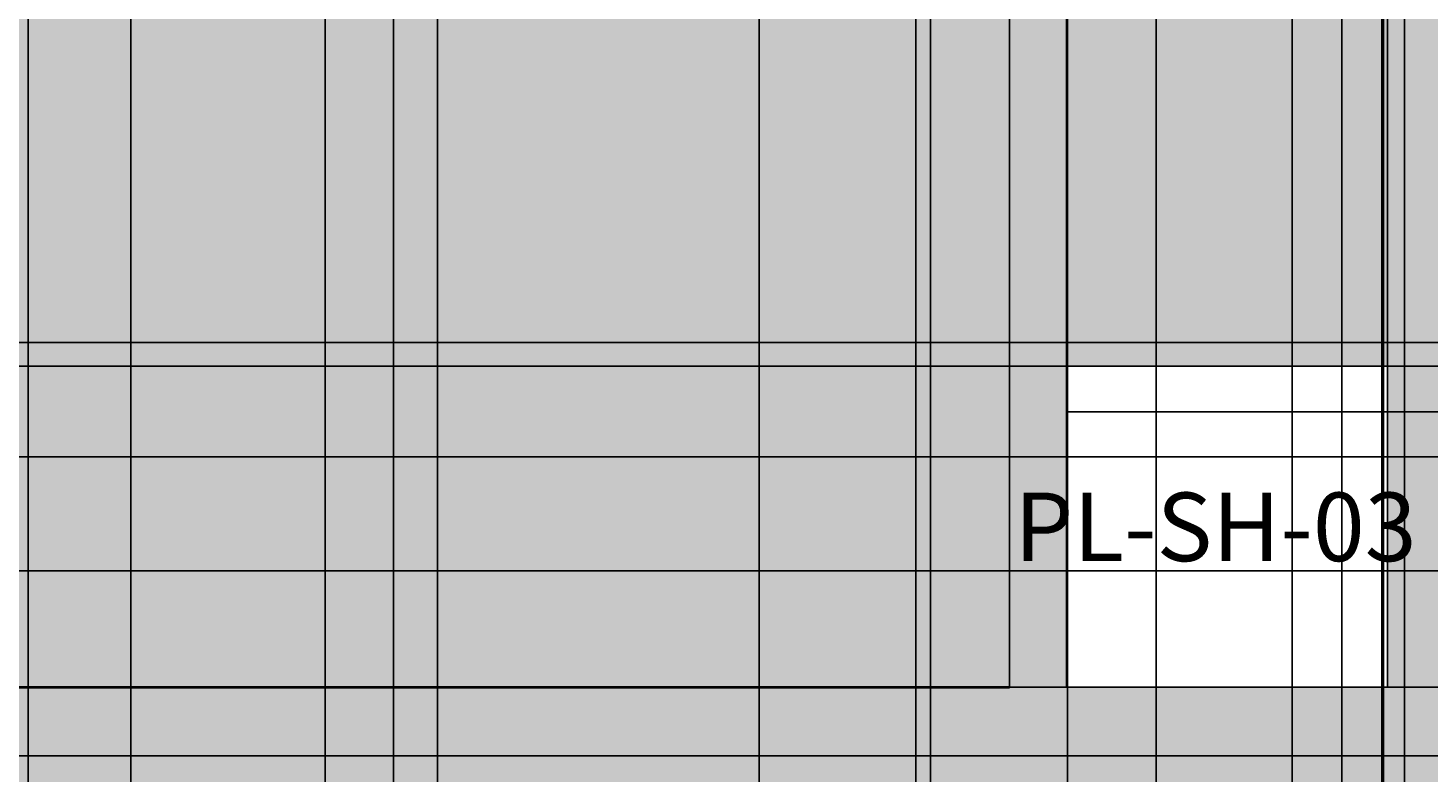
# Model space of a CAD drawing. Units: inches. Extents: x 818 to 1898, y 976 to 2364.
# Tile 91 of 96: x 1591 to 1713, y 2046 to 2111. Entities that reach past the tile are written whole.
import ezdxf

# ---------------------------------------------------------------- set-up
doc = ezdxf.new("R2010")
doc.units = ezdxf.units.IN
doc.header["$LTSCALE"] = 5
doc.header["$MEASUREMENT"] = 0
for name, color, linetype, lineweight in [('A-ANNO-DIMS', 2, 'Continuous', 18), ('A-ANNO-TEXT', 7, 'Continuous', 18), ('A-FLOR-SHFT', 7, 'Continuous', 25), ('A-WALL', 7, 'Continuous', 40)]:
    doc.layers.add(name, color=color, linetype=linetype, lineweight=lineweight)
doc.layers.add('A-WALL-PATT', color=251, linetype='Continuous', lineweight=13, true_color=0x636466)
doc.layers.add('L-PLNT-PATT', color=114, linetype='Continuous', lineweight=9, true_color=0x139b48)
doc.styles.get("Standard").update_dxf_attribs({"font": 'arial.ttf'})
doc.dimstyles.get("Standard").update_dxf_attribs({"dimtxt": 0.18, "dimasz": 0.18, "dimexe": 0.18, "dimexo": 0.0625, "dimgap": 0.09, "dimtad": 0, "dimtih": 1, "dimtoh": 1, "dimdec": 4, "dimzin": 0, "dimdsep": 46, "dimtxsty": 'Standard', "dimcen": 0.09, "dimadec": 0, "dimazin": 0, "dimtfac": 1, "dimtdec": 4, "dimtofl": 0, "dimtmove": 0, "dimatfit": 3, "dimfxl": 1, "dimtolj": 1, "dimtzin": 0, "dimarcsym": 0})

# ---------------------------------------------------------------- blocks, each defined once
blk = doc.blocks.new('*D85')
at = {"layer": 'A-ANNO-DIMS', "color": 0, "lineweight": -2, "ltscale": 5, "transparency": 16777216}
for p, q in [((1258.79, 2053.08), (1897.92, 2053.08)), ((1897.74, 2052.9), (1897.74, 1876.76)), ((1897.74, 1700.26), (1897.74, 1876.4)), ((1258.79, 1700.08), (1897.92, 1700.08))]:
    blk.add_line(p, q, dxfattribs=at)
at = {"layer": 'A-ANNO-DIMS', "color": 0, "ltscale": 5, "transparency": 16777216}
for points in [[(1897.71, 2052.9), (1897.77, 2052.9), (1897.74, 2053.08)], [(1897.71, 1700.26), (1897.77, 1700.26), (1897.74, 1700.08)]]:
    blk.add_solid(points, dxfattribs=at)
at = {"layer": 'Defpoints', "color": 0, "ltscale": 5, "transparency": 16777216}
for p in [(1258.73, 2053.08), (1897.74, 2053.08), (1258.73, 1700.08)]:
    blk.add_point(p, dxfattribs=at)
at = {"layer": 'A-ANNO-DIMS', "color": 0, "ltscale": 5, "transparency": 16777216, "insert": (1897.74, 1876.58), "char_height": 0.18, "attachment_point": 5}
blk.add_mtext('\\A1;353', dxfattribs=at)
blk = doc.blocks.new('*D86')
at = {"layer": 'A-ANNO-DIMS', "color": 0, "lineweight": -2, "ltscale": 5, "transparency": 16777216}
for p, q in [((1258.73, 2053.14), (1258.73, 2363.87)), ((1258.91, 2363.69), (1486.43, 2363.69)), ((1714.55, 2363.69), (1487.02, 2363.69)), ((1714.73, 2053.14), (1714.73, 2363.87))]:
    blk.add_line(p, q, dxfattribs=at)
at = {"layer": 'A-ANNO-DIMS', "color": 0, "ltscale": 5, "transparency": 16777216}
for points in [[(1258.91, 2363.72), (1258.91, 2363.66), (1258.73, 2363.69)], [(1714.55, 2363.72), (1714.55, 2363.66), (1714.73, 2363.69)]]:
    blk.add_solid(points, dxfattribs=at)
at = {"layer": 'Defpoints', "color": 0, "ltscale": 5, "transparency": 16777216}
for p in [(1714.73, 2363.69), (1258.73, 2053.08), (1714.73, 2053.08)]:
    blk.add_point(p, dxfattribs=at)
at = {"layer": 'A-ANNO-DIMS', "color": 0, "ltscale": 5, "transparency": 16777216, "insert": (1486.73, 2363.69), "char_height": 0.18, "attachment_point": 5}
blk.add_mtext('\\A1;456', dxfattribs=at)
blk = doc.blocks.new('*D102')
at = {"layer": 'A-ANNO-DIMS', "color": 0, "lineweight": -2, "ltscale": 5, "transparency": 16777216}
for p, q in [((1565.48, 1071.12), (1565.48, 2363.87)), ((1565.66, 2363.69), (1595.63, 2363.69)), ((1626.39, 2363.69), (1596.42, 2363.69)), ((1626.57, 1071.12), (1626.57, 2363.87))]:
    blk.add_line(p, q, dxfattribs=at)
at = {"layer": 'A-ANNO-DIMS', "color": 0, "ltscale": 5, "transparency": 16777216}
for points in [[(1565.66, 2363.72), (1565.66, 2363.66), (1565.48, 2363.69)], [(1626.39, 2363.72), (1626.39, 2363.66), (1626.57, 2363.69)]]:
    blk.add_solid(points, dxfattribs=at)
at = {"layer": 'Defpoints', "color": 0, "ltscale": 5, "transparency": 16777216}
for p in [(1626.57, 2363.69), (1565.48, 1071.06), (1626.57, 1071.06)]:
    blk.add_point(p, dxfattribs=at)
at = {"layer": 'A-ANNO-DIMS', "color": 0, "ltscale": 5, "transparency": 16777216, "insert": (1596.03, 2363.69), "char_height": 0.18, "attachment_point": 5}
blk.add_mtext('\\A1;61.09', dxfattribs=at)
blk = doc.blocks.new('*D103')
at = {"layer": 'A-ANNO-DIMS', "color": 0, "lineweight": -2, "ltscale": 5, "transparency": 16777216}
for p, q in [((1626.57, 1071.12), (1626.57, 2363.87)), ((1626.75, 2363.69), (1657.7, 2363.69)), ((1689.29, 2363.69), (1658.35, 2363.69)), ((1689.47, 1071.12), (1689.47, 2363.87))]:
    blk.add_line(p, q, dxfattribs=at)
at = {"layer": 'A-ANNO-DIMS', "color": 0, "ltscale": 5, "transparency": 16777216}
for points in [[(1626.75, 2363.72), (1626.75, 2363.66), (1626.57, 2363.69)], [(1689.29, 2363.72), (1689.29, 2363.66), (1689.47, 2363.69)]]:
    blk.add_solid(points, dxfattribs=at)
at = {"layer": 'Defpoints', "color": 0, "ltscale": 5, "transparency": 16777216}
for p in [(1689.47, 2363.69), (1626.57, 1071.06), (1689.47, 1071.06)]:
    blk.add_point(p, dxfattribs=at)
at = {"layer": 'A-ANNO-DIMS', "color": 0, "ltscale": 5, "transparency": 16777216, "insert": (1658.02, 2363.69), "char_height": 0.18, "attachment_point": 5}
blk.add_mtext('\\A1;62.9', dxfattribs=at)
blk = doc.blocks.new('*D104')
at = {"layer": 'A-ANNO-DIMS', "color": 0, "lineweight": -2, "ltscale": 5, "transparency": 16777216}
for p, q in [((1689.47, 1071.12), (1689.47, 2363.87)), ((1689.65, 2363.69), (1717.4, 2363.69)), ((1745.9, 2363.69), (1718.15, 2363.69)), ((1746.08, 1071.12), (1746.08, 2363.87))]:
    blk.add_line(p, q, dxfattribs=at)
at = {"layer": 'A-ANNO-DIMS', "color": 0, "ltscale": 5, "transparency": 16777216}
for points in [[(1689.65, 2363.72), (1689.65, 2363.66), (1689.47, 2363.69)], [(1745.9, 2363.72), (1745.9, 2363.66), (1746.08, 2363.69)]]:
    blk.add_solid(points, dxfattribs=at)
at = {"layer": 'Defpoints', "color": 0, "ltscale": 5, "transparency": 16777216}
for p in [(1746.08, 2363.69), (1689.47, 1071.06), (1746.08, 1071.06)]:
    blk.add_point(p, dxfattribs=at)
at = {"layer": 'A-ANNO-DIMS', "color": 0, "ltscale": 5, "transparency": 16777216, "insert": (1717.78, 2363.69), "char_height": 0.18, "attachment_point": 5}
blk.add_mtext('\\A1;56.61', dxfattribs=at)
blk = doc.blocks.new('*D141')
at = {"layer": 'A-ANNO-DIMS', "color": 0, "lineweight": -2, "ltscale": 5, "transparency": 16777216}
for p, q in [((1218.17, 2083.26), (1897.92, 2083.26)), ((1897.74, 2083.08), (1897.74, 2073.44)), ((1897.74, 2063.44), (1897.74, 2073.08)), ((1198.17, 2063.26), (1897.92, 2063.26))]:
    blk.add_line(p, q, dxfattribs=at)
at = {"layer": 'A-ANNO-DIMS', "color": 0, "ltscale": 5, "transparency": 16777216}
for points in [[(1897.71, 2083.08), (1897.77, 2083.08), (1897.74, 2083.26)], [(1897.71, 2063.44), (1897.77, 2063.44), (1897.74, 2063.26)]]:
    blk.add_solid(points, dxfattribs=at)
at = {"layer": 'Defpoints', "color": 0, "ltscale": 5, "transparency": 16777216}
for p in [(1218.11, 2083.26), (1198.11, 2063.26), (1897.74, 2063.26)]:
    blk.add_point(p, dxfattribs=at)
at = {"layer": 'A-ANNO-DIMS', "color": 0, "ltscale": 5, "transparency": 16777216, "insert": (1897.74, 2073.26), "char_height": 0.18, "attachment_point": 5}
blk.add_mtext('\\A1;20', dxfattribs=at)
blk = doc.blocks.new('*D142')
at = {"layer": 'A-ANNO-DIMS', "color": 0, "lineweight": -2, "ltscale": 5, "transparency": 16777216}
for p, q in [((1208.17, 2073.26), (1897.92, 2073.26)), ((1897.74, 2073.08), (1897.74, 2068.44)), ((1897.74, 2063.44), (1897.74, 2068.08)), ((1198.17, 2063.26), (1897.92, 2063.26))]:
    blk.add_line(p, q, dxfattribs=at)
at = {"layer": 'A-ANNO-DIMS', "color": 0, "ltscale": 5, "transparency": 16777216}
for points in [[(1897.71, 2073.08), (1897.77, 2073.08), (1897.74, 2073.26)], [(1897.71, 2063.44), (1897.77, 2063.44), (1897.74, 2063.26)]]:
    blk.add_solid(points, dxfattribs=at)
at = {"layer": 'Defpoints', "color": 0, "ltscale": 5, "transparency": 16777216}
for p in [(1208.11, 2073.26), (1897.74, 2073.26), (1198.11, 2063.26)]:
    blk.add_point(p, dxfattribs=at)
at = {"layer": 'A-ANNO-DIMS', "color": 0, "ltscale": 5, "transparency": 16777216, "insert": (1897.74, 2068.26), "char_height": 0.18, "attachment_point": 5}
blk.add_mtext('\\A1;10', dxfattribs=at)
blk = doc.blocks.new('*D154')
at = {"layer": 'A-ANNO-DIMS', "color": 0, "lineweight": -2, "ltscale": 5, "transparency": 16777216}
for p, q in [((1701.37, 1290.14), (1701.37, 2363.87)), ((1701.55, 2363.69), (1705.22, 2363.69)), ((1709.19, 2363.69), (1705.52, 2363.69)), ((1709.37, 1298.14), (1709.37, 2363.87))]:
    blk.add_line(p, q, dxfattribs=at)
at = {"layer": 'A-ANNO-DIMS', "color": 0, "ltscale": 5, "transparency": 16777216}
for points in [[(1701.55, 2363.72), (1701.55, 2363.66), (1701.37, 2363.69)], [(1709.19, 2363.72), (1709.19, 2363.66), (1709.37, 2363.69)]]:
    blk.add_solid(points, dxfattribs=at)
at = {"layer": 'Defpoints', "color": 0, "ltscale": 5, "transparency": 16777216}
for p in [(1709.37, 2363.69), (1709.37, 1298.08), (1701.37, 1290.08)]:
    blk.add_point(p, dxfattribs=at)
at = {"layer": 'A-ANNO-DIMS', "color": 0, "ltscale": 5, "transparency": 16777216, "insert": (1705.37, 2363.69), "char_height": 0.18, "attachment_point": 5}
blk.add_mtext('\\A1;8', dxfattribs=at)
blk = doc.blocks.new('*D173')
at = {"layer": 'A-ANNO-DIMS', "color": 0, "lineweight": -2, "ltscale": 5, "transparency": 16777216}
for p, q in [((1622.73, 1463.14), (1622.73, 2363.87)), ((1622.91, 2363.69), (1638.51, 2363.69)), ((1654.55, 2363.69), (1638.94, 2363.69)), ((1654.73, 1463.14), (1654.73, 2363.87))]:
    blk.add_line(p, q, dxfattribs=at)
at = {"layer": 'A-ANNO-DIMS', "color": 0, "ltscale": 5, "transparency": 16777216}
for points in [[(1622.91, 2363.72), (1622.91, 2363.66), (1622.73, 2363.69)], [(1654.55, 2363.72), (1654.55, 2363.66), (1654.73, 2363.69)]]:
    blk.add_solid(points, dxfattribs=at)
at = {"layer": 'Defpoints', "color": 0, "ltscale": 5, "transparency": 16777216}
for p in [(1654.73, 2363.69), (1622.73, 1463.08), (1654.73, 1463.08)]:
    blk.add_point(p, dxfattribs=at)
at = {"layer": 'A-ANNO-DIMS', "color": 0, "ltscale": 5, "transparency": 16777216, "insert": (1638.73, 2363.69), "char_height": 0.18, "attachment_point": 5}
blk.add_mtext('\\A1;32', dxfattribs=at)
blk = doc.blocks.new('*D174')
at = {"layer": 'A-ANNO-DIMS', "color": 0, "lineweight": -2, "ltscale": 5, "transparency": 16777216}
for p, q in [((1616.73, 1416.75), (1616.73, 2363.87)), ((1616.91, 2363.69), (1619.58, 2363.69)), ((1622.55, 2363.69), (1619.87, 2363.69)), ((1622.73, 1416.75), (1622.73, 2363.87))]:
    blk.add_line(p, q, dxfattribs=at)
at = {"layer": 'A-ANNO-DIMS', "color": 0, "ltscale": 5, "transparency": 16777216}
for points in [[(1616.91, 2363.72), (1616.91, 2363.66), (1616.73, 2363.69)], [(1622.55, 2363.72), (1622.55, 2363.66), (1622.73, 2363.69)]]:
    blk.add_solid(points, dxfattribs=at)
at = {"layer": 'Defpoints', "color": 0, "ltscale": 5, "transparency": 16777216}
for p in [(1622.73, 2363.69), (1616.73, 1416.69), (1622.73, 1416.69)]:
    blk.add_point(p, dxfattribs=at)
at = {"layer": 'A-ANNO-DIMS', "color": 0, "ltscale": 5, "transparency": 16777216, "insert": (1619.73, 2363.69), "char_height": 0.18, "attachment_point": 5}
blk.add_mtext('\\A1;6', dxfattribs=at)
blk = doc.blocks.new('*D175')
at = {"layer": 'A-ANNO-DIMS', "color": 0, "lineweight": -2, "ltscale": 5, "transparency": 16777216}
for p, q in [((1559.73, 1647.64), (1559.73, 2363.87)), ((1559.91, 2363.69), (1614.45, 2363.69)), ((1669.55, 2363.69), (1615.01, 2363.69)), ((1669.73, 1647.64), (1669.73, 2363.87))]:
    blk.add_line(p, q, dxfattribs=at)
at = {"layer": 'A-ANNO-DIMS', "color": 0, "ltscale": 5, "transparency": 16777216}
for points in [[(1559.91, 2363.72), (1559.91, 2363.66), (1559.73, 2363.69)], [(1669.55, 2363.72), (1669.55, 2363.66), (1669.73, 2363.69)]]:
    blk.add_solid(points, dxfattribs=at)
at = {"layer": 'Defpoints', "color": 0, "ltscale": 5, "transparency": 16777216}
for p in [(1669.73, 2363.69), (1559.73, 1647.58), (1669.73, 1647.58)]:
    blk.add_point(p, dxfattribs=at)
at = {"layer": 'A-ANNO-DIMS', "color": 0, "ltscale": 5, "transparency": 16777216, "insert": (1614.73, 2363.69), "char_height": 0.18, "attachment_point": 5}
blk.add_mtext('\\A1;110', dxfattribs=at)
blk = doc.blocks.new('*D195')
at = {"layer": 'A-ANNO-DIMS', "color": 0, "lineweight": -2, "ltscale": 5, "transparency": 16777216}
for p, q in [((1681.73, 1379.14), (1681.73, 2363.87)), ((1681.91, 2363.69), (1693.51, 2363.69)), ((1705.55, 2363.69), (1693.95, 2363.69)), ((1705.73, 1355.14), (1705.73, 2363.87))]:
    blk.add_line(p, q, dxfattribs=at)
at = {"layer": 'A-ANNO-DIMS', "color": 0, "ltscale": 5, "transparency": 16777216}
for points in [[(1681.91, 2363.72), (1681.91, 2363.66), (1681.73, 2363.69)], [(1705.55, 2363.72), (1705.55, 2363.66), (1705.73, 2363.69)]]:
    blk.add_solid(points, dxfattribs=at)
at = {"layer": 'Defpoints', "color": 0, "ltscale": 5, "transparency": 16777216}
for p in [(1705.73, 2363.69), (1681.73, 1379.08), (1705.73, 1355.08)]:
    blk.add_point(p, dxfattribs=at)
at = {"layer": 'A-ANNO-DIMS', "color": 0, "ltscale": 5, "transparency": 16777216, "insert": (1693.73, 2363.69), "char_height": 0.18, "attachment_point": 5}
blk.add_mtext('\\A1;24', dxfattribs=at)
blk = doc.blocks.new('*D203')
at = {"layer": 'A-ANNO-DIMS', "color": 0, "lineweight": -2, "ltscale": 5, "transparency": 16777216}
for p, q in [((1599.73, 1876.14), (1599.73, 2363.87)), ((1599.91, 2363.69), (1652.44, 2363.69)), ((1705.55, 2363.69), (1653.01, 2363.69)), ((1705.73, 1876.14), (1705.73, 2363.87))]:
    blk.add_line(p, q, dxfattribs=at)
at = {"layer": 'A-ANNO-DIMS', "color": 0, "ltscale": 5, "transparency": 16777216}
for points in [[(1599.91, 2363.72), (1599.91, 2363.66), (1599.73, 2363.69)], [(1705.55, 2363.72), (1705.55, 2363.66), (1705.73, 2363.69)]]:
    blk.add_solid(points, dxfattribs=at)
at = {"layer": 'Defpoints', "color": 0, "ltscale": 5, "transparency": 16777216}
for p in [(1705.73, 2363.69), (1599.73, 1876.08), (1705.73, 1876.08)]:
    blk.add_point(p, dxfattribs=at)
at = {"layer": 'A-ANNO-DIMS', "color": 0, "ltscale": 5, "transparency": 16777216, "insert": (1652.73, 2363.69), "char_height": 0.18, "attachment_point": 5}
blk.add_mtext('\\A1;106', dxfattribs=at)
blk = doc.blocks.new('*D204')
at = {"layer": 'A-ANNO-DIMS', "color": 0, "lineweight": -2, "ltscale": 5, "transparency": 16777216}
for p, q in [((1714.79, 2053.08), (1897.92, 2053.08)), ((1897.74, 2052.9), (1897.74, 1960.26)), ((1897.74, 1867.26), (1897.74, 1959.9)), ((1705.79, 1867.08), (1897.92, 1867.08))]:
    blk.add_line(p, q, dxfattribs=at)
at = {"layer": 'A-ANNO-DIMS', "color": 0, "ltscale": 5, "transparency": 16777216}
for points in [[(1897.71, 2052.9), (1897.77, 2052.9), (1897.74, 2053.08)], [(1897.71, 1867.26), (1897.77, 1867.26), (1897.74, 1867.08)]]:
    blk.add_solid(points, dxfattribs=at)
at = {"layer": 'Defpoints', "color": 0, "ltscale": 5, "transparency": 16777216}
for p in [(1714.73, 2053.08), (1897.74, 2053.08), (1705.73, 1867.08)]:
    blk.add_point(p, dxfattribs=at)
at = {"layer": 'A-ANNO-DIMS', "color": 0, "ltscale": 5, "transparency": 16777216, "insert": (1897.74, 1960.08), "char_height": 0.18, "attachment_point": 5}
blk.add_mtext('\\A1;186', dxfattribs=at)
blk = doc.blocks.new('*D205')
at = {"layer": 'A-ANNO-DIMS', "color": 0, "lineweight": -2, "ltscale": 5, "transparency": 16777216}
for p, q in [((1590.73, 2044.14), (1590.73, 2363.87)), ((1590.91, 2363.69), (1652.45, 2363.69)), ((1714.55, 2363.69), (1653.01, 2363.69)), ((1714.73, 2053.14), (1714.73, 2363.87))]:
    blk.add_line(p, q, dxfattribs=at)
at = {"layer": 'A-ANNO-DIMS', "color": 0, "ltscale": 5, "transparency": 16777216}
for points in [[(1590.91, 2363.72), (1590.91, 2363.66), (1590.73, 2363.69)], [(1714.55, 2363.72), (1714.55, 2363.66), (1714.73, 2363.69)]]:
    blk.add_solid(points, dxfattribs=at)
at = {"layer": 'Defpoints', "color": 0, "ltscale": 5, "transparency": 16777216}
for p in [(1714.73, 2363.69), (1714.73, 2053.08), (1590.73, 2044.08)]:
    blk.add_point(p, dxfattribs=at)
at = {"layer": 'A-ANNO-DIMS', "color": 0, "ltscale": 5, "transparency": 16777216, "insert": (1652.73, 2363.69), "char_height": 0.18, "attachment_point": 5}
blk.add_mtext('\\A1;124', dxfattribs=at)
blk = doc.blocks.new('*D213')
at = {"layer": 'A-ANNO-DIMS', "color": 0, "lineweight": -2, "ltscale": 5, "transparency": 16777216}
for p, q in [((1709.23, 1962.1), (1709.23, 2363.87)), ((1709.41, 2363.69), (1710.08, 2363.69)), ((1711.05, 2363.69), (1710.37, 2363.69)), ((1711.23, 1962.1), (1711.23, 2363.87))]:
    blk.add_line(p, q, dxfattribs=at)
at = {"layer": 'A-ANNO-DIMS', "color": 0, "ltscale": 5, "transparency": 16777216}
for points in [[(1709.41, 2363.72), (1709.41, 2363.66), (1709.23, 2363.69)], [(1711.05, 2363.72), (1711.05, 2363.66), (1711.23, 2363.69)]]:
    blk.add_solid(points, dxfattribs=at)
at = {"layer": 'Defpoints', "color": 0, "ltscale": 5, "transparency": 16777216}
for p in [(1711.23, 2363.69), (1709.23, 1962.03), (1711.23, 1962.03)]:
    blk.add_point(p, dxfattribs=at)
at = {"layer": 'A-ANNO-DIMS', "color": 0, "ltscale": 5, "transparency": 16777216, "insert": (1710.23, 2363.69), "char_height": 0.18, "attachment_point": 5}
blk.add_mtext('\\A1;2', dxfattribs=at)
blk = doc.blocks.new('*D230')
at = {"layer": 'A-ANNO-DIMS', "color": 0, "lineweight": -2, "ltscale": 5, "transparency": 16777216}
for p, q in [((1668.44, 2044.14), (1668.44, 2363.87)), ((1668.62, 2363.69), (1686.69, 2363.69)), ((1705.55, 2363.69), (1687.48, 2363.69)), ((1705.73, 2044.14), (1705.73, 2363.87))]:
    blk.add_line(p, q, dxfattribs=at)
at = {"layer": 'A-ANNO-DIMS', "color": 0, "ltscale": 5, "transparency": 16777216}
for points in [[(1668.62, 2363.72), (1668.62, 2363.66), (1668.44, 2363.69)], [(1705.55, 2363.72), (1705.55, 2363.66), (1705.73, 2363.69)]]:
    blk.add_solid(points, dxfattribs=at)
at = {"layer": 'Defpoints', "color": 0, "ltscale": 5, "transparency": 16777216}
for p in [(1705.73, 2363.69), (1668.44, 2044.08), (1705.73, 2044.08)]:
    blk.add_point(p, dxfattribs=at)
at = {"layer": 'A-ANNO-DIMS', "color": 0, "ltscale": 5, "transparency": 16777216, "insert": (1687.08, 2363.69), "char_height": 0.18, "attachment_point": 5}
blk.add_mtext('\\A1;37.28', dxfattribs=at)
blk = doc.blocks.new('*D259')
at = {"layer": 'A-ANNO-DIMS', "color": 0, "lineweight": -2, "ltscale": 5, "transparency": 16777216}
for p, q in [((1681.64, 2053.14), (1681.64, 2363.87)), ((1681.82, 2363.69), (1695.29, 2363.69)), ((1709.55, 2363.69), (1696.08, 2363.69)), ((1709.73, 2077.25), (1709.73, 2363.87))]:
    blk.add_line(p, q, dxfattribs=at)
at = {"layer": 'A-ANNO-DIMS', "color": 0, "ltscale": 5, "transparency": 16777216}
for points in [[(1681.82, 2363.72), (1681.82, 2363.66), (1681.64, 2363.69)], [(1709.55, 2363.72), (1709.55, 2363.66), (1709.73, 2363.69)]]:
    blk.add_solid(points, dxfattribs=at)
at = {"layer": 'Defpoints', "color": 0, "ltscale": 5, "transparency": 16777216}
for p in [(1709.73, 2363.69), (1709.73, 2077.19), (1681.64, 2053.08)]:
    blk.add_point(p, dxfattribs=at)
at = {"layer": 'A-ANNO-DIMS', "color": 0, "ltscale": 5, "transparency": 16777216, "insert": (1695.68, 2363.69), "char_height": 0.18, "attachment_point": 5}
blk.add_mtext('\\A1;28.08', dxfattribs=at)
blk = doc.blocks.new('*D260')
at = {"layer": 'A-ANNO-DIMS', "color": 0, "lineweight": -2, "ltscale": 5, "transparency": 16777216}
for p, q in [((1709.79, 2077.19), (1897.92, 2077.19)), ((1897.74, 2077.01), (1897.74, 2065.31)), ((1897.74, 2053.26), (1897.74, 2064.95)), ((1709.79, 2053.08), (1897.92, 2053.08))]:
    blk.add_line(p, q, dxfattribs=at)
at = {"layer": 'A-ANNO-DIMS', "color": 0, "ltscale": 5, "transparency": 16777216}
for points in [[(1897.71, 2077.01), (1897.77, 2077.01), (1897.74, 2077.19)], [(1897.71, 2053.26), (1897.77, 2053.26), (1897.74, 2053.08)]]:
    blk.add_solid(points, dxfattribs=at)
at = {"layer": 'Defpoints', "color": 0, "ltscale": 5, "transparency": 16777216}
for p in [(1709.73, 2077.19), (1897.74, 2077.19), (1709.73, 2053.08)]:
    blk.add_point(p, dxfattribs=at)
at = {"layer": 'A-ANNO-DIMS', "color": 0, "ltscale": 5, "transparency": 16777216, "insert": (1897.74, 2065.13), "char_height": 0.18, "attachment_point": 5}
blk.add_mtext('\\A1;24.11', dxfattribs=at)
blk = doc.blocks.new('*D261')
at = {"layer": 'A-ANNO-DIMS', "color": 0, "lineweight": -2, "ltscale": 5, "transparency": 16777216}
for p, q in [((1676.64, 2081.25), (1676.64, 2363.87)), ((1676.82, 2363.69), (1678.99, 2363.69)), ((1681.46, 2363.69), (1679.29, 2363.69)), ((1681.64, 2077.25), (1681.64, 2363.87))]:
    blk.add_line(p, q, dxfattribs=at)
at = {"layer": 'A-ANNO-DIMS', "color": 0, "ltscale": 5, "transparency": 16777216}
for points in [[(1676.82, 2363.72), (1676.82, 2363.66), (1676.64, 2363.69)], [(1681.46, 2363.72), (1681.46, 2363.66), (1681.64, 2363.69)]]:
    blk.add_solid(points, dxfattribs=at)
at = {"layer": 'Defpoints', "color": 0, "ltscale": 5, "transparency": 16777216}
for p in [(1681.64, 2363.69), (1676.64, 2081.19), (1681.64, 2077.19)]:
    blk.add_point(p, dxfattribs=at)
at = {"layer": 'A-ANNO-DIMS', "color": 0, "ltscale": 5, "transparency": 16777216, "insert": (1679.14, 2363.69), "char_height": 0.18, "attachment_point": 5}
blk.add_mtext('\\A1;5', dxfattribs=at)
blk = doc.blocks.new('*D266')
at = {"layer": 'A-ANNO-DIMS', "color": 0, "lineweight": -2, "ltscale": 5, "transparency": 16777216}
for p, q in [((1780.44, 2053.08), (818.03, 2053.08)), ((818.21, 2052.9), (818.21, 2050.26)), ((818.21, 2047.26), (818.21, 2049.9)), ((1780.44, 2047.08), (818.03, 2047.08))]:
    blk.add_line(p, q, dxfattribs=at)
at = {"layer": 'A-ANNO-DIMS', "color": 0, "ltscale": 5, "transparency": 16777216}
for points in [[(818.18, 2052.9), (818.24, 2052.9), (818.21, 2053.08)], [(818.18, 2047.26), (818.24, 2047.26), (818.21, 2047.08)]]:
    blk.add_solid(points, dxfattribs=at)
at = {"layer": 'Defpoints', "color": 0, "ltscale": 5, "transparency": 16777216}
for p in [(1780.5, 2053.08), (818.21, 2047.08), (1780.5, 2047.08)]:
    blk.add_point(p, dxfattribs=at)
at = {"layer": 'A-ANNO-DIMS', "color": 0, "ltscale": 5, "transparency": 16777216, "insert": (818.21, 2050.08), "char_height": 0.18, "attachment_point": 5}
blk.add_mtext('\\A1;6', dxfattribs=at)
blk = doc.blocks.new('*D282')
at = {"layer": 'A-ANNO-DIMS', "color": 0, "lineweight": -2, "ltscale": 5, "transparency": 16777216}
for p, q in [((1422.08, 2081.19), (1897.92, 2081.19)), ((1897.74, 2081.01), (1897.74, 1884.32)), ((1897.74, 1687.26), (1897.74, 1883.95)), ((1463.79, 1687.08), (1897.92, 1687.08))]:
    blk.add_line(p, q, dxfattribs=at)
at = {"layer": 'A-ANNO-DIMS', "color": 0, "ltscale": 5, "transparency": 16777216}
for points in [[(1897.71, 2081.01), (1897.77, 2081.01), (1897.74, 2081.19)], [(1897.71, 1687.26), (1897.77, 1687.26), (1897.74, 1687.08)]]:
    blk.add_solid(points, dxfattribs=at)
at = {"layer": 'Defpoints', "color": 0, "ltscale": 5, "transparency": 16777216}
for p in [(1422.02, 2081.19), (1897.74, 2081.19), (1463.73, 1687.08)]:
    blk.add_point(p, dxfattribs=at)
at = {"layer": 'A-ANNO-DIMS', "color": 0, "ltscale": 5, "transparency": 16777216, "insert": (1897.74, 1884.13), "char_height": 0.18, "attachment_point": 5}
blk.add_mtext('\\A1;394.1', dxfattribs=at)

msp = doc.modelspace()

# ---------------------------------------------------------------- hatches: boundary and pattern name
at = {"layer": 'A-WALL-PATT', "ltscale": 5}
h = msp.add_hatch(color=256, dxfattribs=at)
h.dxf.hatch_style = 1
h.paths.add_polyline_path([(1267.7252, 1928.9218), (1258.7251, 1928.9218), (1258.7251, 1913.6401), (1250.3029, 1913.6401), (1250.3029, 1878.3919), (1258.7251, 1878.3919), (1258.7251, 1862.9652), (1267.7252, 1862.9652)])
h.paths.add_polyline_path([(1267.7252, 1814.9652), (1258.7251, 1814.9652), (1258.7251, 1755.3321), (1267.7252, 1755.3321)])
h.paths.add_polyline_path([(1463.7251, 1696.0782), (1267.7252, 1696.0782), (1267.7252, 1707.3321), (1258.7251, 1707.3321), (1258.7251, 1700.0782), (1251.9333, 1700.0782), (1251.9333, 1687.0782), (1463.7251, 1687.0782)])
h.paths.add_polyline_path([(1714.7251, 1717.3178), (1705.7251, 1717.3178), (1705.7251, 1696.0782), (1599.7251, 1696.0782), (1599.7251, 1790.0782), (1705.7251, 1790.0782), (1705.7251, 1785.6125), (1714.7251, 1785.6125), (1714.7251, 1827.2125), (1705.7251, 1827.2125), (1705.7251, 1802.0782), (1599.7251, 1802.0782), (1599.7251, 1867.0782), (1705.7251, 1867.0782), (1705.7251, 1857.2125), (1714.7251, 1857.2125), (1714.7251, 1930.0316), (1741.8409, 1930.0316), (1741.8409, 1935.0316), (1714.7251, 1935.0316), (1714.7251, 1957.0338), (1741.8409, 1957.0338), (1741.8409, 1962.0338), (1714.7251, 1962.0338), (1705.7251, 1962.0338), (1705.7251, 1948.0782), (1599.7251, 1948.0782), (1599.7251, 1981.0782), (1590.7251, 1981.0782), (1590.7251, 1941.0782), (1620.7252, 1941.0782), (1705.7251, 1941.0782), (1705.7251, 1876.0782), (1599.7251, 1876.0782), (1599.7251, 1911.0782), (1590.7251, 1911.0782), (1590.7251, 1876.0782), (1429.2252, 1876.0782), (1429.2252, 1867.0782), (1511.7252, 1867.0782), (1528.593, 1867.0782), (1595.7252, 1867.0782), (1595.7252, 1773.0782), (1520.7252, 1773.0782), (1520.7252, 1837.5823), (1532.593, 1837.5823), (1532.593, 1867.0782), (1528.593, 1867.0782), (1528.593, 1841.5823), (1511.7252, 1841.5823), (1511.7252, 1744.9714), (1520.7252, 1744.9714), (1520.7252, 1761.0782), (1595.7252, 1761.0782), (1595.7252, 1696.0782), (1520.7252, 1696.0782), (1520.7252, 1716.0454), (1511.7252, 1716.0454), (1511.7252, 1696.0782), (1511.7252, 1687.0782), (1714.7251, 1687.0782)])
h.paths.add_polyline_path([(1714.7251, 2053.0782), (1714.7251, 2081.1881), (1709.7251, 2081.1881), (1709.7251, 2053.0782), (1681.6446, 2053.0782), (1681.6446, 2081.1881), (1676.6446, 2081.1881), (1676.6446, 2053.0782), (1538.5155, 2053.0782), (1538.5155, 2044.0782), (1590.7251, 2044.0782), (1590.7251, 2011.0782), (1599.7251, 2011.0782), (1599.7251, 2044.0782), (1705.7251, 2044.0782), (1705.7251, 2014.5114), (1714.7251, 2014.5114)])
h.paths.add_polyline_path([(1485.1216, 2053.0782), (1422.02, 2053.0782), (1422.02, 2081.1881), (1413.02, 2081.1881), (1413.02, 2053.0782), (1399.6356, 2053.0782), (1399.6356, 2081.1881), (1390.6356, 2081.1881), (1390.6356, 2053.0782), (1388.0315, 2053.0782), (1388.0315, 2044.0782), (1416.2743, 2044.0782), (1485.1216, 2044.0782)])
h.paths.add_polyline_path([(1330.305, 2053.0782), (1258.7251, 2053.0782), (1258.7251, 2019.2871), (1267.7252, 2019.2871), (1267.7252, 2044.0782), (1330.305, 2044.0782)])
h.paths.add_polyline_path([(1258.7251, 2053.0782), (1214.6577, 2053.0782), (1214.6577, 2044.0782), (1258.7251, 2044.0782)])
h.paths.add_polyline_path([(1214.6577, 2053.0782), (1180.349, 2053.0782), (1180.349, 2044.0782), (1214.6577, 2044.0782)])
h.paths.add_polyline_path([(1714.7251, 1639.5782), (1741.8409, 1639.5782), (1741.8409, 1643.5782), (1714.7251, 1643.5782), (1714.7251, 1649.9029), (1705.7251, 1649.9029), (1705.7251, 1600.0782), (1477.7252, 1600.0782), (1477.7252, 1591.0782), (1520.7252, 1591.0782), (1616.7251, 1591.0782), (1616.7251, 1416.6857), (1622.7251, 1416.6857), (1622.7251, 1463.0782), (1624.7252, 1463.0782), (1624.7252, 1467.0782), (1622.7251, 1467.0782), (1622.7251, 1591.0782), (1705.7251, 1591.0782), (1705.7251, 1545.0782), (1714.7251, 1545.0782), (1741.8409, 1545.0782), (1741.8409, 1549.0782), (1714.7251, 1549.0782), (1714.7251, 1593.9175), (1737.8409, 1593.9175), (1737.8409, 1597.9175), (1714.7251, 1597.9175)])
h.paths.add_polyline_path([(1674.9024, 2060.7419), (1714.7045, 2060.7419), (1714.7045, 2073.1061), (1674.9024, 2073.1061)], flags=25)
h.paths.add_polyline_path([(1394.5468, 2061.6618), (1422.2344, 2061.6618), (1422.2344, 2074.0261), (1394.5468, 2074.0261)], flags=24)
at = {"layer": 'L-PLNT-PATT', "ltscale": 5}
h = msp.add_hatch(color=256, dxfattribs=at)
h.dxf.hatch_style = 1
h.paths.add_polyline_path([(1789.7173, 2205.9709), (1083.7252, 2205.9709), (1083.7252, 2083.2623), (1218.1114, 2083.2623), (1218.1114, 2053.0782), (1390.6356, 2053.0782), (1390.6356, 2081.1881), (1399.6356, 2081.1881), (1413.02, 2081.1881), (1422.02, 2081.1881), (1422.02, 2053.0782), (1676.6446, 2053.0782), (1676.6446, 2081.1881), (1714.7251, 2081.1881), (1714.7251, 2081.6235), (1789.7173, 2081.6235)])
h.paths.add_polyline_path([(1388.6037, 2145.2461), (1388.6037, 2122.3767), (1373.4756, 2122.3767), (1373.4756, 2145.2461)], flags=16)
h.paths.add_polyline_path([(1408.6922, 2145.2461), (1423.8203, 2145.2461), (1423.8203, 2122.3767), (1408.6922, 2122.3767)], flags=16)
h.paths.add_polyline_path([(1353.3871, 2155.7839), (1353.3871, 2122.3767), (1338.259, 2122.3767), (1338.259, 2155.7839)], flags=16)
h.paths.add_polyline_path([(1443.9089, 2158.4222), (1459.037, 2158.4222), (1459.037, 2122.3767), (1443.9089, 2122.3767)], flags=16)
h.paths.add_polyline_path([(1318.1705, 2145.2461), (1318.1705, 2122.3767), (1303.0424, 2122.3767), (1303.0424, 2145.2461)], flags=16)
h.paths.add_polyline_path([(1479.1255, 2145.2461), (1494.2536, 2145.2461), (1494.2536, 2122.3767), (1479.1255, 2122.3767)], flags=16)
h.paths.add_polyline_path([(1282.9539, 2145.2461), (1282.9539, 2122.3767), (1267.8258, 2122.3767), (1267.8258, 2145.2461)], flags=16)
h.paths.add_polyline_path([(1514.3421, 2145.2461), (1529.4702, 2145.2461), (1529.4702, 2122.3767), (1514.3421, 2122.3767)], flags=16)
h.paths.add_polyline_path([(1247.7373, 2159.4296), (1247.7373, 2122.3767), (1232.6091, 2122.3767), (1232.6091, 2159.4296)], flags=16)
h.paths.add_polyline_path([(1549.5587, 2156.9246), (1564.6868, 2156.9246), (1564.6868, 2122.3767), (1549.5587, 2122.3767)], flags=16)
h.paths.add_polyline_path([(1212.5206, 2145.2461), (1212.5206, 2122.3767), (1197.3925, 2122.3767), (1197.3925, 2145.2461)], flags=16)
h.paths.add_polyline_path([(1584.7753, 2145.2461), (1599.9034, 2145.2461), (1599.9034, 2122.3767), (1584.7753, 2122.3767)], flags=16)
h.paths.add_polyline_path([(1185.1073, 2104.7786), (1190.6407, 2104.7786), (1185.1073, 2098.2505), (1179.5738, 2104.7786)], flags=16)
h.paths.add_polyline_path([(1619.9919, 2145.2461), (1635.1201, 2145.2461), (1635.1201, 2122.3767), (1619.9919, 2122.3767)], flags=16)
h.paths.add_polyline_path([(1655.2086, 2156.1761), (1670.3367, 2156.1761), (1670.3367, 2122.3767), (1655.2086, 2122.3767)], flags=16)
h.paths.add_polyline_path([(1686.5992, 2145.2461), (1701.7273, 2145.2461), (1701.7273, 2122.3767), (1686.5992, 2122.3767)], flags=16)
h.paths.add_polyline_path([(1715.7616, 2145.2461), (1730.8897, 2145.2461), (1730.8897, 2122.3767), (1715.7616, 2122.3767)], flags=16)
h.paths.add_polyline_path([(1753.1652, 2145.2461), (1776.3312, 2145.2461), (1776.3312, 2115.6891), (1753.1652, 2115.6891)], flags=16)
h.paths.add_polyline_path([(1191.4331, 2146.5159), (1176.7891, 2146.5159), (1176.7891, 2134.1516), (1191.4331, 2134.1516)], flags=24)

# ---------------------------------------------------------------- linework, layer by layer
at = {"layer": 'A-FLOR-SHFT'}
for p, q in [((1676.6446, 2081.1881), (1714.7251, 2081.1881)), ((1676.6446, 2053.0782), (1676.6446, 2081.1881)), ((1681.6446, 2053.0782), (1681.6446, 2081.1881)), ((1709.7251, 2053.0782), (1709.7251, 2081.1881)), ((1681.6446, 2077.1881), (1709.7251, 2077.1881)), ((1681.6446, 2053.0782), (1709.7251, 2053.0782))]:
    msp.add_line(p, q, dxfattribs=at)
at = {"layer": 'A-WALL'}
msp.add_line((1422.02, 2053.0782), (1676.6446, 2053.0782), dxfattribs=at)

# ---------------------------------------------------------------- texts
at = {"layer": 'A-ANNO-TEXT', "ltscale": 5, "insert": (1677.049, 2070.1205), "char_height": 6, "attachment_point": 1}
msp.add_mtext_dynamic_manual_height_columns('PL-SH-03', width=118.992422, gutter_width=1, heights=[0], dxfattribs=at)

# ---------------------------------------------------------------- dimensions: what is measured, and where the dimension line sits
at = {"layer": 'A-ANNO-DIMS', "ltscale": 5}
for base, p1, p2, override, picture, middle in [((1714.7251, 2363.6929), (1258.7251, 2053.0782), (1714.7251, 2053.0782), {"dimdec": 0, "dimlfac": 1, "dimrnd": 0, "dimzin": 0, "dimdsep": 46, "dimlunit": 2}, '*D86', (1486.7251, 2363.6929)), ((1669.7251, 2363.6929), (1559.7251, 1647.5782), (1669.7251, 1647.5782), {"dimdec": 0, "dimlfac": 1, "dimrnd": 0, "dimzin": 0, "dimdsep": 46, "dimlunit": 2}, '*D175', (1614.7251, 2363.6929)), ((1626.5748, 2363.6929), (1565.4835, 1071.0552), (1626.5748, 1071.0552), {"dimdec": 2, "dimlfac": 1, "dimrnd": 0, "dimzin": 0, "dimdsep": 46, "dimlunit": 2}, '*D102', (1596.0291, 2363.6929)), ((1714.7251, 2363.6929), (1590.7251, 2044.0782), (1714.7251, 2053.0782), {"dimdec": 0, "dimlfac": 1, "dimrnd": 0, "dimzin": 0, "dimdsep": 46, "dimlunit": 2}, '*D205', (1652.7251, 2363.6929)), ((1705.7251, 2363.6929), (1599.7251, 1876.0782), (1705.7251, 1876.0782), {"dimdec": 0, "dimlfac": 1, "dimrnd": 0, "dimzin": 0, "dimdsep": 46, "dimlunit": 2}, '*D203', (1652.7251, 2363.6929)), ((1622.7251, 2363.6929), (1616.7251, 1416.6857), (1622.7251, 1416.6857), {"dimdec": 0, "dimlfac": 1, "dimrnd": 0, "dimzin": 0, "dimdsep": 46, "dimlunit": 2}, '*D174', (1619.7251, 2363.6929)), ((1654.7251, 2363.6929), (1622.7251, 1463.0782), (1654.7251, 1463.0782), {"dimdec": 0, "dimlfac": 1, "dimrnd": 0, "dimzin": 0, "dimdsep": 46, "dimlunit": 2}, '*D173', (1638.7251, 2363.6929)), ((1689.4714, 2363.6929), (1626.5748, 1071.0552), (1689.4714, 1071.0552), {"dimdec": 1, "dimlfac": 1, "dimrnd": 0, "dimzin": 0, "dimdsep": 46, "dimlunit": 2}, '*D103', (1658.0231, 2363.6929)), ((1705.7251, 2363.6929), (1668.4429, 2044.0782), (1705.7251, 2044.0782), {"dimdec": 2, "dimlfac": 1, "dimrnd": 0, "dimzin": 0, "dimdsep": 46, "dimlunit": 2}, '*D230', (1687.084, 2363.6929)), ((1681.6446, 2363.6929), (1676.6446, 2081.1881), (1681.6446, 2077.1881), {"dimdec": 0, "dimlfac": 1, "dimrnd": 0, "dimzin": 0, "dimdsep": 46, "dimlunit": 2}, '*D261', (1679.1446, 2363.6929)), ((1709.7251, 2363.6929), (1681.6446, 2053.0782), (1709.7251, 2077.1881), {"dimdec": 2, "dimlfac": 1, "dimrnd": 0, "dimzin": 0, "dimdsep": 46, "dimlunit": 2}, '*D259', (1695.6849, 2363.6929)), ((1705.7251, 2363.6929), (1681.7251, 1379.0782), (1705.7251, 1355.0782), {"dimdec": 0, "dimlfac": 1, "dimrnd": 0, "dimzin": 0, "dimdsep": 46, "dimlunit": 2}, '*D195', (1693.7251, 2363.6929)), ((1746.0831, 2363.6929), (1689.4714, 1071.0552), (1746.0831, 1071.0552), {"dimdec": 2, "dimlfac": 1, "dimrnd": 0, "dimzin": 0, "dimdsep": 46, "dimlunit": 2}, '*D104', (1717.7772, 2363.6929)), ((1709.3688, 2363.6929), (1701.3688, 1290.0782), (1709.3688, 1298.0782), {"dimdec": 0, "dimlfac": 1, "dimrnd": 0, "dimzin": 0, "dimdsep": 46, "dimlunit": 2}, '*D154', (1705.3688, 2363.6929)), ((1711.2251, 2363.6929), (1709.2251, 1962.0338), (1711.2251, 1962.0338), {"dimdec": 0, "dimlfac": 1, "dimrnd": 0, "dimzin": 0, "dimdsep": 46, "dimlunit": 2}, '*D213', (1710.2251, 2363.6929))]:
    dim = msp.add_linear_dim(base=base, p1=p1, p2=p2, dimstyle='Standard', override=override, dxfattribs=at)
    dim.commit()
    dim.dimension.update_dxf_attribs({"geometry": picture, "text_midpoint": middle})
for base, p1, p2, override, picture, middle in [((1897.736, 2063.2623), (1218.1114, 2083.2623), (1198.1114, 2063.2623), {"dimdec": 0, "dimlfac": 1, "dimrnd": 0, "dimzin": 0, "dimdsep": 46, "dimlunit": 2}, '*D141', (1897.736, 2073.2623)), ((1897.736, 2081.1881), (1463.7251, 1687.0782), (1422.02, 2081.1881), {"dimdec": 1, "dimlfac": 1, "dimrnd": 0, "dimzin": 0, "dimdsep": 46, "dimlunit": 2}, '*D282', (1897.736, 1884.1332)), ((1897.736, 2077.1881), (1709.7251, 2053.0782), (1709.7251, 2077.1881), {"dimdec": 2, "dimlfac": 1, "dimrnd": 0, "dimzin": 0, "dimdsep": 46, "dimlunit": 2}, '*D260', (1897.736, 2065.1332)), ((1897.736, 2073.2623), (1198.1114, 2063.2623), (1208.1114, 2073.2623), {"dimdec": 0, "dimlfac": 1, "dimrnd": 0, "dimzin": 0, "dimdsep": 46, "dimlunit": 2}, '*D142', (1897.736, 2068.2623)), ((818.2059, 2047.0782), (1780.5019, 2053.0782), (1780.5019, 2047.0782), {"dimdec": 0, "dimlfac": 1, "dimrnd": 0, "dimzin": 0, "dimdsep": 46, "dimlunit": 2}, '*D266', (818.2059, 2050.0782)), ((1897.736, 2053.0782), (1258.7251, 1700.0782), (1258.7251, 2053.0782), {"dimdec": 0, "dimlfac": 1, "dimrnd": 0, "dimzin": 0, "dimdsep": 46, "dimlunit": 2}, '*D85', (1897.736, 1876.5782)), ((1897.736, 2053.0782), (1705.7251, 1867.0782), (1714.7251, 2053.0782), {"dimdec": 0, "dimlfac": 1, "dimrnd": 0, "dimzin": 0, "dimdsep": 46, "dimlunit": 2}, '*D204', (1897.736, 1960.0782))]:
    dim = msp.add_linear_dim(base=base, p1=p1, p2=p2, angle=90, dimstyle='Standard', override=override, dxfattribs=at)
    dim.commit()
    dim.dimension.update_dxf_attribs({"geometry": picture, "text_midpoint": middle})

doc.saveas('drawing.dxf')
